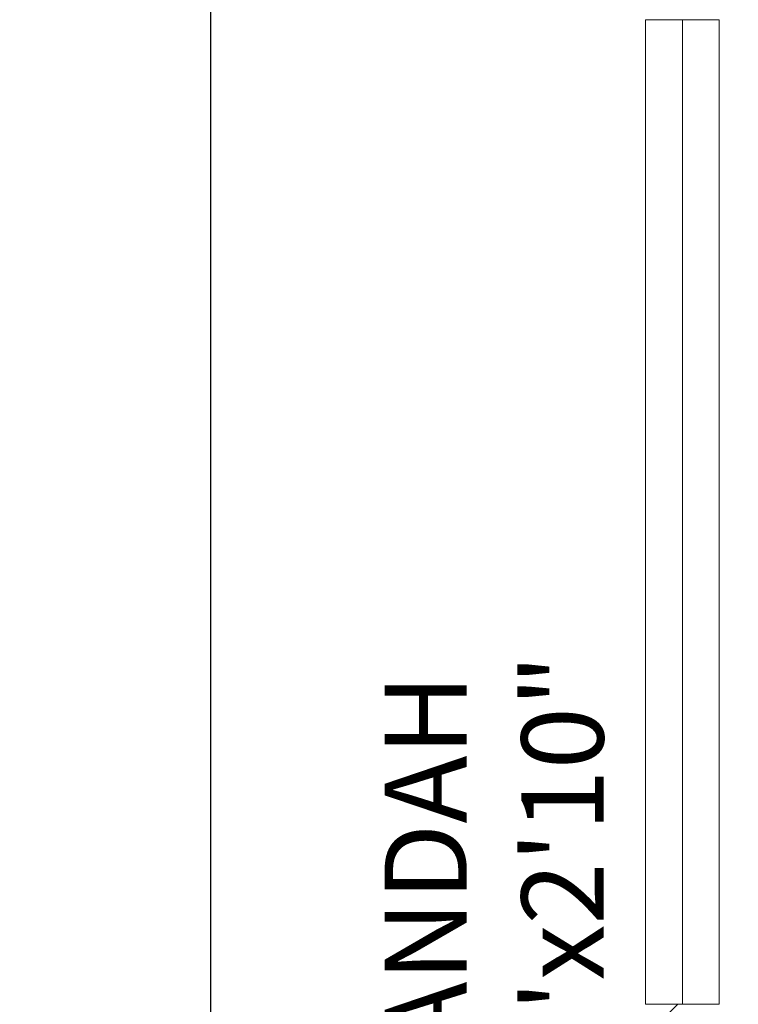
# Model space of a CAD drawing. Units: inches. Extents: x 1885 to 2748, y 783 to 2421.
# Tile 31 of 117: x 1969 to 2013, y 1443 to 1503. Entities that reach past the tile are written whole.
import ezdxf

# ---------------------------------------------------------------- set-up
doc = ezdxf.new("R2010")
doc.units = ezdxf.units.IN
for name, color, linetype, lineweight in [('A-ANNO-DIMS', 2, 'Continuous', 18), ('A-AREA-IDEN', 7, 'Continuous', 18), ('A-FLOR-BALC', 7, 'Continuous', 25), ('A-GLAZ', 181, 'Continuous', 18)]:
    doc.layers.add(name, color=color, linetype=linetype, lineweight=lineweight)
doc.layers.add('A-WALL-PATT', color=85, linetype='Continuous', lineweight=13, true_color=0x58ba48)
doc.styles.get("Standard").update_dxf_attribs({"font": 'arial.ttf'})
doc.dimstyles.get("Standard").update_dxf_attribs({"dimtxt": 0.18, "dimasz": 0.18, "dimexe": 0.18, "dimexo": 0.0625, "dimgap": 0.09, "dimtad": 0, "dimtih": 1, "dimtoh": 1, "dimdec": 4, "dimzin": 0, "dimdsep": 46, "dimtxsty": 'Standard', "dimcen": 0.09, "dimadec": 0, "dimazin": 0, "dimtfac": 1, "dimtdec": 4, "dimtofl": 0, "dimtmove": 0, "dimatfit": 3, "dimfxl": 1, "dimtolj": 1, "dimtzin": 0, "dimarcsym": 0})

# ---------------------------------------------------------------- blocks, each defined once
blk = doc.blocks.new('WIN-60-ALT')
for p, q in [((0.004, 59.998), (4.504, 59.998)), ((0.004, 59.998), (0.004, -0.002)), ((4.504, 59.998), (2.254, 59.998)), ((2.254, 59.998), (2.254, -0.002)), ((4.504, -0.002), (4.504, 59.998)), ((4.504, -0.002), (0.004, -0.002)), ((2.254, -0.002), (4.504, -0.002))]:
    blk.add_line(p, q)
blk = doc.blocks.new('*D45')
at = {"layer": 'A-ANNO-DIMS', "color": 0, "lineweight": -2, "transparency": 16777216}
for p, q in [((1980.711, 1524.006), (1902.844, 1524.006)), ((1903.024, 1523.826), (1903.024, 1290.937)), ((1903.024, 1057.686), (1903.024, 1290.574)), ((1971.211, 1057.506), (1902.844, 1057.506))]:
    blk.add_line(p, q, dxfattribs=at)
at = {"layer": 'A-ANNO-DIMS', "color": 0, "transparency": 16777216}
for points in [[(1902.994, 1523.826), (1903.054, 1523.826), (1903.024, 1524.006)], [(1902.994, 1057.686), (1903.054, 1057.686), (1903.024, 1057.506)]]:
    blk.add_solid(points, dxfattribs=at)
at = {"layer": 'Defpoints', "color": 0, "transparency": 16777216}
for p in [(1903.024, 1524.006), (1980.774, 1524.006), (1971.274, 1057.506)]:
    blk.add_point(p, dxfattribs=at)
at = {"layer": 'A-ANNO-DIMS', "color": 0, "transparency": 16777216, "insert": (1903.024, 1290.756), "char_height": 0.18, "attachment_point": 5}
blk.add_mtext('\\A1;466.5', dxfattribs=at)

msp = doc.modelspace()

# ---------------------------------------------------------------- hatches: boundary and pattern name
at = {"layer": 'A-WALL-PATT'}
h = msp.add_hatch(dxfattribs=at)
h.set_pattern_fill('ANSI32', color=256)
h.paths.add_polyline_path([(2007.772, 2318.006), (1980.774, 2318.006), (1980.774, 2281.215), (1985.274, 2281.215), (1985.274, 2313.506), (2007.772, 2313.506), (2007.772, 2315.756)])
h.paths.add_polyline_path([(2094.324, 2318.006), (2067.772, 2318.006), (2067.772, 2313.506), (2094.324, 2313.506), (2094.324, 2315.756)])
h.paths.add_polyline_path([(2131.367, 2315.756), (2131.367, 2318.006), (2131.189, 2318.006), (2112.609, 2318.006), (2112.609, 2313.506), (2117.274, 2313.506), (2117.274, 2255.201), (2121.774, 2255.201), (2121.774, 2313.506), (2131.367, 2313.506)])
h.paths.add_polyline_path([(2190.512, 2318.006), (2155.367, 2318.006), (2155.367, 2313.506), (2169.774, 2313.506), (2169.774, 2229.506), (2121.774, 2229.506), (2121.774, 2233.451), (2119.524, 2233.451), (2117.274, 2233.451), (2117.274, 2201.101), (2121.774, 2201.101), (2121.774, 2225.006), (2169.774, 2225.006), (2169.774, 2165.006), (2306.274, 2165.006), (2306.274, 2066.006), (2310.774, 2066.006), (2344.274, 2066.006), (2486.274, 2066.006), (2486.274, 1886.006), (2483.02, 1886.006), (2483.02, 1881.506), (2486.274, 1881.506), (2486.274, 1880.678), (2490.774, 1880.678), (2490.774, 2070.506), (2344.274, 2070.506), (2310.774, 2070.506), (2310.774, 2165.006), (2310.774, 2173.636), (2308.524, 2173.636), (2306.274, 2173.636), (2306.274, 2169.506), (2174.274, 2169.506), (2174.274, 2313.506), (2190.512, 2313.506), (2190.512, 2315.756)])
h.paths.add_polyline_path([(1985.274, 2221.215), (1980.774, 2221.215), (1980.774, 2165.006), (1992.774, 2165.006), (1992.774, 2141.927), (1997.274, 2141.927), (1997.274, 2165.006), (2117.274, 2165.006), (2117.274, 2163.126), (2121.774, 2163.126), (2121.774, 2172.734), (2119.524, 2172.734), (2117.274, 2172.734), (2117.274, 2169.506), (1985.274, 2169.506)])
h.paths.add_polyline_path([(1997.274, 2105.927), (1992.774, 2105.927), (1992.774, 2070.506), (2016.774, 2070.506), (2016.774, 2059.123), (2019.024, 2059.123), (2021.274, 2059.123), (2021.274, 2070.506), (2117.274, 2070.506), (2117.274, 2022.506), (2114.423, 2022.506), (2114.423, 2018.006), (2123.627, 2018.006), (2123.627, 2020.256), (2123.627, 2022.506), (2121.774, 2022.506), (2121.774, 2142.587), (2119.524, 2142.587), (2117.274, 2142.587), (2117.274, 2075.006), (1997.274, 2075.006)])
h.paths.add_polyline_path([(2092.029, 2020.256), (2092.029, 2022.506), (2021.274, 2022.506), (2021.274, 2035.123), (2016.774, 2035.123), (2016.774, 2018.006), (2016.774, 1978.784), (2021.274, 1978.784), (2021.274, 2018.006), (2092.029, 2018.006)])
h.paths.add_polyline_path([(2260.938, 2022.506), (2153.105, 2022.506), (2153.105, 2020.256), (2153.105, 2018.006), (2155.274, 2018.006), (2155.274, 1886.006), (2107.629, 1886.006), (2107.629, 1881.506), (2182.911, 1881.506), (2182.911, 1883.756), (2182.911, 1886.006), (2159.774, 1886.006), (2159.774, 2018.006), (2260.938, 2018.006), (2260.938, 2020.256)])
h.paths.add_polyline_path([(2047.629, 1883.756), (2047.629, 1886.006), (2021.274, 1886.006), (2021.274, 1918.784), (2019.024, 1918.784), (2016.774, 1918.784), (2016.774, 1881.506), (2047.629, 1881.506)])
h.paths.add_polyline_path([(2306.361, 1883.756), (2306.361, 1886.006), (2296.274, 1886.006), (2296.274, 1982.006), (2316.535, 1982.006), (2316.535, 1984.256), (2316.535, 1986.506), (2296.274, 1986.506), (2296.274, 2022.506), (2289.276, 2022.506), (2289.276, 2018.006), (2291.774, 2018.006), (2291.774, 1886.006), (2242.911, 1886.006), (2242.911, 1881.506), (2306.361, 1881.506)], flags=17)
h.paths.add_polyline_path([(1985.274, 1843.006), (2021.6, 1843.006), (2021.534, 1845.441), (2021.477, 1847.506), (1980.774, 1847.506), (1980.774, 1809.446), (1985.274, 1809.446)])
h.paths.add_polyline_path([(2131.482, 1845.256), (2131.482, 1847.506), (2081.534, 1847.506), (2081.534, 1843.006), (2117.274, 1843.006), (2117.274, 1784.147), (2119.524, 1784.147), (2121.774, 1784.147), (2121.774, 1843.006), (2131.482, 1843.006)])
h.paths.add_polyline_path([(2203.886, 1847.506), (2155.482, 1847.506), (2155.482, 1843.006), (2169.774, 1843.006), (2169.774, 1759.006), (2121.774, 1759.006), (2121.774, 1761.457), (2117.274, 1761.457), (2117.274, 1730.429), (2121.774, 1730.429), (2121.774, 1754.506), (2177.421, 1754.506), (2177.421, 1756.756), (2177.421, 1759.006), (2174.274, 1759.006), (2174.274, 1843.006), (2203.886, 1843.006)])
h.paths.add_polyline_path([(2335.554, 1845.256), (2335.554, 1847.506), (2239.886, 1847.506), (2239.886, 1843.006), (2306.274, 1843.006), (2306.274, 1759.006), (2199.486, 1759.006), (2199.486, 1754.506), (2310.774, 1754.506), (2310.774, 1843.006), (2335.554, 1843.006)])
h.paths.add_polyline_path([(2348.774, 2022.506), (2344.274, 2022.506), (2344.274, 1986.506), (2341.681, 1986.506), (2341.681, 1982.006), (2344.274, 1982.006), (2344.274, 1886.006), (2330.361, 1886.006), (2330.361, 1881.506), (2361.627, 1881.506), (2361.627, 1883.756), (2361.627, 1886.006), (2348.774, 1886.006)], flags=17)
h.paths.add_polyline_path([(2283.251, 2315.756), (2283.251, 2318.006), (2238.512, 2318.006), (2238.512, 2313.506), (2283.251, 2313.506)], flags=17)
h.paths.add_polyline_path([(2363.274, 2348.006), (2388.677, 2348.006), (2388.677, 2350.256), (2388.677, 2352.506), (2358.774, 2352.506), (2358.774, 2348.006), (2358.774, 2318.006), (2344.481, 2318.006), (2344.481, 2313.506), (2358.774, 2313.506), (2358.774, 2229.506), (2310.774, 2229.506), (2310.774, 2231.952), (2306.274, 2231.952), (2306.274, 2205.611), (2310.774, 2205.611), (2310.774, 2225.006), (2358.774, 2225.006), (2358.774, 2211.506), (2452.329, 2211.506), (2452.329, 2213.756), (2452.329, 2216.006), (2363.274, 2216.006), (2363.274, 2318.006)])
h.paths.add_polyline_path([(2310.774, 2313.506), (2320.481, 2313.506), (2320.481, 2315.756), (2320.481, 2318.006), (2302.728, 2318.006), (2302.728, 2313.506), (2306.274, 2313.506), (2306.274, 2251.076), (2310.774, 2251.076)], flags=17)
h.paths.add_polyline_path([(2490.774, 2352.506), (2486.274, 2352.506), (2448.677, 2352.506), (2448.677, 2348.006), (2486.274, 2348.006), (2486.274, 2318.006), (2486.274, 2216.006), (2481.78, 2216.006), (2481.78, 2211.506), (2486.274, 2211.506), (2486.274, 2165.006), (2493.289, 2165.006), (2493.289, 2167.256), (2493.289, 2169.506), (2490.774, 2169.506), (2490.774, 2313.506), (2494.429, 2313.506), (2494.429, 2318.006), (2490.774, 2318.006)])
h.paths.add_polyline_path([(2534.653, 2318.006), (2515.691, 2318.006), (2515.691, 2313.506), (2534.653, 2313.506), (2534.653, 2315.756)])
h.paths.add_polyline_path([(2618.274, 2318.006), (2594.653, 2318.006), (2594.653, 2313.506), (2613.774, 2313.506), (2613.774, 2281.706), (2618.274, 2281.706)])
h.paths.add_polyline_path([(2618.274, 2221.706), (2613.774, 2221.706), (2613.774, 2169.506), (2554.019, 2169.506), (2554.019, 2165.006), (2613.774, 2165.006), (2613.774, 2152.878), (2618.274, 2152.878)])
h.paths.add_polyline_path([(2618.274, 2128.878), (2616.024, 2128.878), (2613.774, 2128.878), (2613.774, 2117.006), (2529.774, 2117.006), (2529.774, 2165.006), (2532.848, 2165.006), (2532.848, 2169.506), (2522.867, 2169.506), (2522.867, 2165.006), (2525.274, 2165.006), (2525.274, 2117.006), (2525.274, 2112.506), (2525.274, 2108.576), (2529.774, 2108.576), (2529.774, 2112.506), (2613.774, 2112.506), (2613.774, 2080.19), (2618.274, 2080.19)])
h.paths.add_polyline_path([(2618.274, 2044.19), (2616.024, 2044.19), (2613.774, 2044.19), (2613.774, 2015.506), (2529.774, 2015.506), (2529.774, 2088.582), (2527.524, 2088.582), (2525.274, 2088.582), (2525.274, 2011.006), (2613.774, 2011.006), (2613.774, 1956.755), (2618.274, 1956.755)])
h.paths.add_polyline_path([(2618.274, 1881.506), (2618.274, 1896.755), (2613.774, 1896.755), (2613.774, 1881.506), (2613.774, 1847.506), (2592.715, 1847.506), (2592.715, 1843.006), (2613.774, 1843.006), (2613.774, 1765.006), (2613.774, 1760.506), (2609.621, 1760.506), (2609.621, 1756.006), (2613.774, 1756.006), (2613.774, 1660.006), (2608.544, 1660.006), (2608.544, 1655.506), (2613.774, 1655.506), (2613.774, 1508.158), (2618.274, 1508.158)])
h.paths.add_polyline_path([(2565.774, 1843.006), (2568.997, 1843.006), (2568.997, 1847.506), (2490.774, 1847.506), (2490.774, 1849.7), (2488.524, 1849.7), (2486.274, 1849.7), (2486.274, 1847.506), (2477.274, 1847.506), (2477.274, 1838.506), (2477.274, 1821.493), (2486.274, 1821.493), (2486.274, 1838.506), (2561.274, 1838.506), (2561.274, 1765.006), (2486.274, 1765.006), (2486.274, 1786.157), (2477.274, 1786.157), (2477.274, 1765.006), (2477.274, 1756.006), (2486.274, 1756.006), (2565.774, 1756.006), (2585.621, 1756.006), (2585.621, 1758.256), (2585.621, 1760.506), (2565.774, 1760.506), (2565.774, 1765.006)])
h.paths.add_polyline_path([(2486.274, 1651.006), (2561.274, 1651.006), (2561.274, 1567.006), (2486.274, 1567.006), (2486.274, 1591.321), (2477.274, 1591.321), (2477.274, 1567.006), (2477.274, 1558.006), (2477.274, 1555.439), (2481.774, 1555.439), (2481.774, 1558.006), (2568.653, 1558.006), (2568.653, 1560.256), (2568.653, 1562.506), (2565.774, 1562.506), (2565.774, 1655.506), (2584.544, 1655.506), (2584.544, 1657.756), (2584.544, 1660.006), (2565.774, 1660.006), (2486.274, 1660.006), (2477.274, 1660.006), (2477.274, 1651.006), (2477.274, 1632.989), (2486.274, 1632.989)])
h.paths.add_polyline_path([(2449.967, 1883.756), (2449.967, 1886.006), (2421.627, 1886.006), (2421.627, 1881.506), (2449.967, 1881.506)], flags=17)
h.paths.add_polyline_path([(2447.274, 1847.506), (2395.554, 1847.506), (2395.554, 1843.006), (2442.774, 1843.006), (2442.774, 1809.27), (2447.274, 1809.27)])
h.paths.add_polyline_path([(1985.274, 1749.446), (1980.774, 1749.446), (1980.774, 1694.504), (1985.274, 1694.504), (1985.274, 1694.506), (1986.897, 1694.506), (1986.897, 1697.78), (1986.897, 1699.006), (1985.274, 1699.006)])
h.paths.add_polyline_path([(2152.774, 1699.006), (2121.774, 1699.006), (2121.774, 1703.668), (2119.524, 1703.668), (2117.274, 1703.668), (2117.274, 1699.006), (2009.219, 1699.006), (2009.219, 1694.506), (2148.274, 1694.506), (2148.274, 1692.631), (2152.774, 1692.631)])
h.paths.add_polyline_path([(2016.274, 1694.506), (2011.774, 1694.506), (2011.774, 1558.006), (2040.806, 1558.006), (2040.806, 1560.256), (2040.806, 1562.506), (2016.274, 1562.506)])
h.paths.add_polyline_path([(2152.774, 1663.017), (2150.524, 1663.017), (2148.274, 1663.017), (2148.274, 1562.506), (2100.806, 1562.506), (2100.806, 1558.006), (2165.119, 1558.006), (2165.119, 1560.256), (2165.119, 1562.506), (2152.774, 1562.506), (2152.774, 1610.506), (2224.774, 1610.506), (2224.774, 1607.99), (2229.274, 1607.99), (2229.274, 1615.006), (2152.774, 1615.006)])
h.paths.add_polyline_path([(2238.613, 1560.256), (2238.613, 1562.506), (2229.274, 1562.506), (2229.274, 1588.756), (2227.024, 1588.763), (2224.774, 1588.771), (2224.774, 1562.506), (2189.119, 1562.506), (2189.119, 1558.006), (2238.613, 1558.006)])
h.paths.add_polyline_path([(2336.024, 1560.256), (2336.024, 1562.506), (2310.774, 1562.506), (2310.774, 1656.347), (2308.524, 1656.347), (2306.274, 1656.347), (2306.274, 1562.506), (2286.613, 1562.506), (2286.613, 1558.006), (2336.024, 1558.006)])
h.paths.add_polyline_path([(2447.274, 1690.968), (2445.024, 1690.968), (2442.774, 1690.968), (2442.774, 1687.006), (2306.274, 1687.006), (2306.274, 1680.75), (2310.774, 1680.75), (2310.774, 1682.506), (2442.774, 1682.506), (2442.774, 1562.506), (2396.024, 1562.506), (2396.024, 1558.006), (2447.274, 1558.006)])
h.paths.add_polyline_path([(2447.274, 1749.27), (2445.024, 1749.27), (2442.774, 1749.27), (2442.774, 1717.232), (2447.274, 1717.232)])
h.paths.add_polyline_path([(2044.674, 1521.756), (2044.674, 1524.006), (2007.274, 1524.006), (2007.274, 1503.49), (2009.524, 1503.49), (2011.774, 1503.49), (2011.774, 1519.506), (2044.674, 1519.506)])
h.paths.add_polyline_path([(2177.969, 1521.756), (2177.969, 1524.006), (2104.674, 1524.006), (2104.674, 1519.506), (2145.774, 1519.506), (2145.774, 1387.506), (2143.37, 1387.506), (2143.37, 1383.006), (2251.585, 1383.006), (2251.585, 1385.256), (2251.585, 1387.506), (2150.274, 1387.506), (2150.274, 1519.506), (2177.969, 1519.506)])
h.paths.add_polyline_path([(2298.704, 1524.006), (2237.969, 1524.006), (2237.969, 1519.506), (2282.274, 1519.506), (2282.274, 1387.506), (2279.683, 1387.506), (2279.683, 1383.006), (2286.774, 1383.006), (2286.774, 1419.006), (2312.451, 1419.006), (2312.451, 1421.256), (2312.451, 1423.506), (2286.774, 1423.506), (2286.774, 1519.506), (2298.704, 1519.506), (2298.704, 1521.722)], flags=17)
h.paths.add_polyline_path([(2361.897, 1521.756), (2361.897, 1524.006), (2322.704, 1524.006), (2322.704, 1519.506), (2334.774, 1519.506), (2334.774, 1423.506), (2331.93, 1423.506), (2331.93, 1419.006), (2334.774, 1419.006), (2334.774, 1387.506), (2334.774, 1383.228), (2339.274, 1383.228), (2339.274, 1387.506), (2339.274, 1519.506), (2361.897, 1519.506)], flags=17)
h.paths.add_polyline_path([(2447.274, 1521.756), (2447.274, 1524.006), (2421.897, 1524.006), (2421.897, 1519.506), (2447.274, 1519.506)], flags=17)
h.paths.add_polyline_path([(2481.774, 1529.6), (2479.524, 1529.6), (2477.274, 1529.6), (2477.274, 1524.006), (2474.489, 1524.006), (2474.489, 1519.506), (2477.274, 1519.506), (2477.274, 1334.506), (2296.774, 1334.506), (2296.774, 1240.506), (2160.274, 1240.506), (2160.274, 1180.506), (2112.274, 1180.506), (2112.274, 1207.692), (2110.024, 1207.692), (2107.774, 1207.692), (2107.774, 1171.609), (2112.274, 1171.609), (2112.274, 1176.006), (2160.274, 1176.006), (2160.274, 1092.006), (2144.221, 1092.006), (2144.221, 1087.506), (2189.497, 1087.506), (2189.497, 1089.756), (2189.497, 1092.006), (2164.774, 1092.006), (2164.774, 1236.006), (2296.774, 1236.006), (2296.774, 1231.912), (2301.274, 1231.912), (2301.274, 1330.006), (2481.774, 1330.006), (2481.774, 1387.506)])
h.paths.add_polyline_path([(2618.274, 1448.158), (2613.774, 1448.158), (2613.774, 1382.506), (2529.774, 1382.506), (2525.274, 1382.506), (2525.274, 1307.062), (2529.774, 1307.062), (2529.774, 1378.006), (2613.774, 1378.006), (2613.774, 1354.988), (2618.274, 1354.988)])
h.paths.add_polyline_path([(2618.274, 1318.988), (2613.774, 1318.988), (2613.774, 1281.006), (2529.774, 1281.006), (2529.774, 1283.786), (2527.524, 1283.786), (2525.274, 1283.786), (2525.274, 1228.506), (2516.794, 1228.506), (2516.794, 1224.006), (2533.484, 1224.006), (2533.484, 1226.256), (2533.484, 1228.506), (2529.774, 1228.506), (2529.774, 1276.506), (2613.774, 1276.506), (2613.774, 1266.02), (2618.274, 1266.02)])
h.paths.add_polyline_path([(2618.274, 1134.964), (2613.774, 1134.964), (2613.774, 1092.006), (2594.545, 1092.006), (2594.545, 1087.506), (2618.274, 1087.506)])
h.paths.add_polyline_path([(2534.545, 1092.006), (2509.765, 1092.006), (2509.765, 1087.506), (2534.545, 1087.506), (2534.545, 1089.756)])
h.paths.add_polyline_path([(2481.274, 1224.006), (2484.117, 1224.006), (2484.117, 1226.256), (2484.117, 1228.506), (2476.774, 1228.506), (2476.774, 1198.506), (2471.61, 1198.506), (2471.61, 1194.006), (2476.774, 1194.006), (2476.774, 1062.006), (2436.894, 1062.006), (2436.894, 1057.506), (2476.774, 1057.506), (2481.274, 1057.506), (2481.274, 1062.006), (2481.274, 1087.506), (2485.354, 1087.506), (2485.354, 1089.756), (2485.354, 1092.006), (2481.274, 1092.006), (2481.274, 1117.506)])
h.paths.add_polyline_path([(2439.898, 1198.506), (2349.274, 1198.506), (2349.274, 1194.006), (2349.274, 1180.506), (2301.274, 1180.506), (2301.274, 1201.896), (2299.024, 1201.896), (2296.774, 1201.896), (2296.774, 1172.335), (2299.024, 1172.335), (2301.274, 1172.335), (2301.274, 1176.006), (2349.274, 1176.006), (2349.274, 1092.006), (2334.452, 1092.006), (2334.452, 1087.506), (2349.274, 1087.506), (2349.274, 1057.506), (2353.774, 1057.506), (2376.894, 1057.506), (2376.894, 1059.756), (2376.894, 1062.006), (2353.774, 1062.006), (2353.774, 1087.506), (2353.774, 1180.506), (2353.774, 1194.006), (2439.898, 1194.006), (2439.898, 1196.256)])
h.paths.add_polyline_path([(2270.596, 1089.756), (2270.596, 1092.006), (2249.497, 1092.006), (2249.497, 1087.506), (2270.596, 1087.506)], flags=17)
h.paths.add_polyline_path([(2310.452, 1092.006), (2301.274, 1092.006), (2301.274, 1153.292), (2296.774, 1153.292), (2296.774, 1092.006), (2293.786, 1092.006), (2293.786, 1087.506), (2310.452, 1087.506), (2310.452, 1089.756)], flags=17)
h.paths.add_polyline_path([(2112.274, 1150.328), (2110.024, 1150.328), (2107.774, 1150.328), (2107.774, 1092.006), (2104.465, 1092.006), (2104.465, 1087.506), (2120.221, 1087.506), (2120.221, 1089.756), (2120.221, 1092.006), (2112.274, 1092.006)])
h.paths.add_polyline_path([(2082.172, 1092.006), (2058.144, 1092.006), (2058.144, 1087.506), (2082.172, 1087.506), (2082.172, 1089.756)])
h.paths.add_polyline_path([(1975.774, 1145.638), (1971.274, 1145.638), (1971.274, 1087.506), (1980.774, 1087.506), (1998.144, 1087.506), (1998.144, 1089.756), (1998.144, 1092.006), (1985.274, 1092.006), (1975.774, 1092.006)])
h.paths.add_polyline_path([(2112.274, 1244.385), (2110.024, 1244.385), (2107.774, 1244.385), (2107.774, 1240.506), (1992.274, 1240.506), (1992.274, 1271.008), (1987.774, 1271.008), (1987.774, 1240.506), (1980.774, 1240.506), (1975.774, 1240.506), (1971.274, 1240.506), (1971.274, 1205.638), (1975.774, 1205.638), (1975.774, 1236.006), (2107.774, 1236.006), (2107.774, 1233.444), (2112.274, 1233.444), (2112.274, 1236.006)])
h.paths.add_polyline_path([(2112.274, 1383.006), (2114.783, 1383.006), (2114.783, 1385.256), (2114.783, 1387.506), (2102.476, 1387.506), (2102.476, 1383.006), (2107.774, 1383.006), (2107.774, 1335.006), (2011.774, 1335.006), (2011.774, 1349.939), (2007.274, 1349.939), (2007.274, 1335.006), (1987.774, 1335.006), (1987.774, 1330.506), (1987.774, 1307.008), (1992.274, 1307.008), (1992.274, 1330.506), (2007.274, 1330.506), (2107.774, 1330.506), (2107.774, 1264.711), (2112.274, 1264.711)])
h.paths.add_polyline_path([(2077.857, 1387.506), (2011.774, 1387.506), (2011.774, 1390.036), (2009.524, 1390.036), (2007.274, 1390.036), (2007.274, 1373.939), (2011.774, 1373.939), (2011.774, 1383.006), (2077.857, 1383.006)])
h.paths.add_polyline_path([(2011.774, 1443.49), (2007.274, 1443.49), (2007.274, 1410.248), (2011.774, 1410.248)])

# ---------------------------------------------------------------- linework, layer by layer
at = {"layer": 'A-FLOR-BALC'}
msp.add_line((1980.774, 1524.006), (1980.774, 1383.006), dxfattribs=at)

# ---------------------------------------------------------------- block references
at = {"layer": 'A-GLAZ', "extrusion": (0, 0, -1), "zscale": -1}
msp.add_blockref('WIN-60-ALT', (-2011.777, 1443.493), dxfattribs=at)

# ---------------------------------------------------------------- texts
at = {"layer": 'A-AREA-IDEN', "insert": (1991.383, 1428.461), "char_height": 5, "attachment_point": 1, "rotation": 90}
msp.add_mtext_dynamic_manual_height_columns('VERANDAH\\P12\'0"x2\'10"', width=104.66534, gutter_width=12.5, heights=[0], dxfattribs=at)

# ---------------------------------------------------------------- dimensions: what is measured, and where the dimension line sits
at = {"layer": 'A-ANNO-DIMS'}
dim = msp.add_linear_dim(base=(1903.024, 1524.006), p1=(1971.274, 1057.506), p2=(1980.774, 1524.006), angle=90, dimstyle='Standard', override={"dimdec": 1, "dimlfac": 1, "dimrnd": 0, "dimzin": 0, "dimdsep": 46, "dimlunit": 2}, dxfattribs=at)
dim.commit()
dim.dimension.update_dxf_attribs({"geometry": '*D45', "text_midpoint": (1903.024, 1290.756)})

doc.saveas('drawing.dxf')
